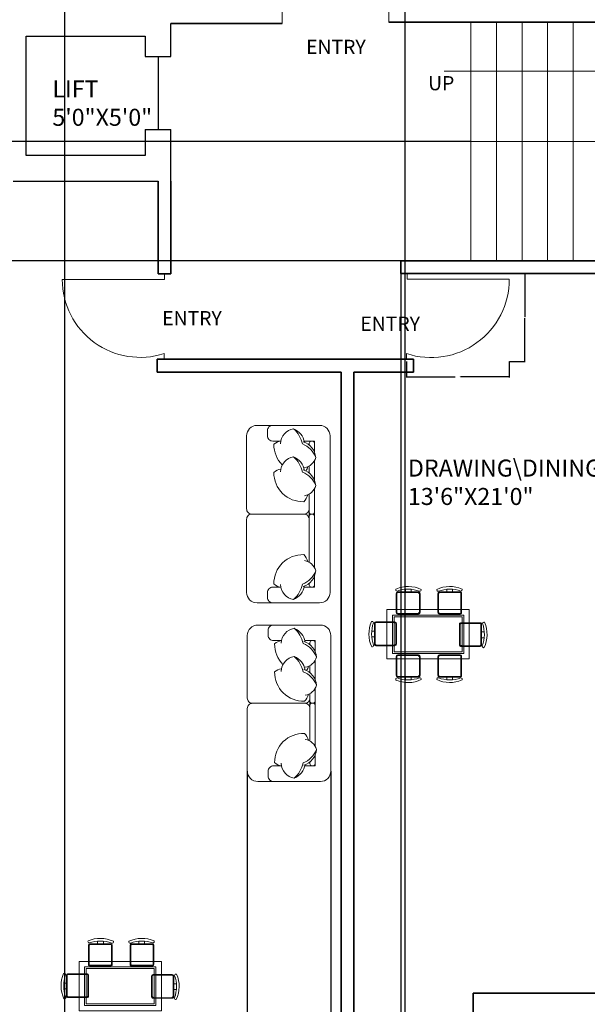
# Model space of a CAD drawing. Units: inches. Extents: x 1088 to 1703, y 668 to 1875.
# Tile 3 of 45: x 1302 to 1502, y 1069 to 1416. Entities that reach past the tile are written whole.
import ezdxf

# ---------------------------------------------------------------- set-up
doc = ezdxf.new("R2010")
doc.units = ezdxf.units.IN
for name, color, linetype, lineweight in [('A-ANNO-DIMS', 2, 'Continuous', 18), ('A-ANNO-SYMB', 7, 'Continuous', 18), ('A-ANNO-TEXT', 7, 'Continuous', 18), ('A-AREA-IDEN', 7, 'Continuous', 18), ('A-DOOR', 4, 'Continuous', 18), ('A-FLOR-EVTR', 5, 'Continuous', 25), ('A-FLOR-STRS', 7, 'Continuous', 18), ('A-FURN', 8, 'Continuous', 13), ('A-WALL', 7, 'Continuous', 35)]:
    doc.layers.add(name, color=color, linetype=linetype, lineweight=lineweight)
doc.styles.get("Standard").update_dxf_attribs({"font": 'arial.ttf'})
doc.dimstyles.get("Standard").update_dxf_attribs({"dimtxt": 0.18, "dimasz": 0.18, "dimexe": 0.18, "dimexo": 0.0625, "dimgap": 0.09, "dimtad": 0, "dimtih": 1, "dimtoh": 1, "dimdec": 4, "dimzin": 0, "dimdsep": 46, "dimtxsty": 'Standard', "dimcen": 0.09, "dimadec": 0, "dimazin": 0, "dimtfac": 1, "dimtdec": 4, "dimtofl": 0, "dimtmove": 0, "dimatfit": 3, "dimfxl": 1, "dimtolj": 1, "dimtzin": 0, "dimarcsym": 0})

# ---------------------------------------------------------------- blocks, each defined once
blk = doc.blocks.new('TABLE-DINING-RECT')
for points in [[(0, 17.41), (29.01, 17.41), (29.01, 0), (0, 0)], [(1.93, 15.47), (27.08, 15.47), (27.08, 1.93), (1.93, 1.93)], [(2.51, 14.89), (26.5, 14.89), (26.5, 2.51), (2.51, 2.51)]]:
    blk.add_lwpolyline(points, close=True)
blk = doc.blocks.new('CHAIR-DINING')
for points in [[(7.77, 8.29, 0.414214), (7.26, 8.81), (0.51, 8.81, 0.414214), (0, 8.29), (0, 0.96, 0.414214), (0.51, 0.44), (7.26, 0.44, 0.414214), (7.77, 0.96), (7.77, 8.29)], [(8.09, 8.52, -0.175809), (8.03, 0.62, 0.578392), (8.69, 0.02, 0.214524), (8.81, 8.94, 0.552014), (8.09, 8.52, -0.065079)], [(7.77, 3.53), (8.7, 3.53, -0.064759)]]:
    blk.add_lwpolyline(points, format="xyb")
blk.add_lwpolyline([(7.54, 8.29), (7.54, 1.19, -0.414214), (7.03, 0.68), (0.74, 0.68, -0.414214), (0.23, 1.19), (0.23, 8.29, -0.512069), (0.74, 8.58), (7.03, 8.58, -0.512069)], format="xyb", close=True)
blk.add_lwpolyline([(8.72, 5.59), (7.77, 5.59)])
blk = doc.blocks.new('DOOR-SWING-36')
for p, q in [((36.2, 30.23), (36.2, 28.23)), ((36, 2), (0, 2)), ((36, 0), (36, 2))]:
    blk.add_line(p, q)
blk.add_arc((27.61, 2), 27.61, 71.8583, 180)
blk = doc.blocks.new('*D26')
at = {"layer": 'A-ANNO-DIMS', "color": 0, "lineweight": -2, "transparency": 16777216}
for p, q in [((1437.89, 1295.51), (1437.89, 1289.96)), ((1474.09, 1295.51), (1474.09, 1289.96)), ((1438.07, 1290.14), (1455.06, 1290.14)), ((1473.91, 1290.14), (1456.93, 1290.14))]:
    blk.add_line(p, q, dxfattribs=at)
at = {"layer": 'A-ANNO-DIMS', "color": 0, "transparency": 16777216}
for points in [[(1438.07, 1290.17), (1438.07, 1290.11), (1437.89, 1290.14)], [(1473.91, 1290.17), (1473.91, 1290.11), (1474.09, 1290.14)]]:
    blk.add_solid(points, dxfattribs=at)
at = {"layer": 'Defpoints', "color": 0, "transparency": 16777216}
for p in [(1437.89, 1295.57), (1474.09, 1295.57), (1437.89, 1290.14)]:
    blk.add_point(p, dxfattribs=at)
at = {"layer": 'A-ANNO-DIMS', "color": 0, "transparency": 16777216, "insert": (1455.99, 1290.14), "char_height": 0.18, "attachment_point": 5}
blk.add_mtext('\\A1;DOOR 36 TYP.', dxfattribs=at)
blk = doc.blocks.new('*D27')
at = {"layer": 'A-ANNO-DIMS', "color": 0, "lineweight": -2, "transparency": 16777216}
for p, q in [((1474.16, 1326.56), (1479.71, 1326.56)), ((1479.53, 1326.38), (1479.53, 1311.25)), ((1479.53, 1295.75), (1479.53, 1310.88)), ((1474.16, 1295.57), (1479.71, 1295.57))]:
    blk.add_line(p, q, dxfattribs=at)
at = {"layer": 'A-ANNO-DIMS', "color": 0, "transparency": 16777216}
for points in [[(1479.5, 1326.38), (1479.56, 1326.38), (1479.53, 1326.56)], [(1479.5, 1295.75), (1479.56, 1295.75), (1479.53, 1295.57)]]:
    blk.add_solid(points, dxfattribs=at)
at = {"layer": 'Defpoints', "color": 0, "transparency": 16777216}
for p in [(1474.1, 1326.56), (1474.09, 1295.57), (1479.53, 1295.57)]:
    blk.add_point(p, dxfattribs=at)
at = {"layer": 'A-ANNO-DIMS', "color": 0, "transparency": 16777216, "insert": (1479.53, 1311.06), "char_height": 0.18, "attachment_point": 5}
blk.add_mtext('\\A1;31 TYP.', dxfattribs=at)
blk = doc.blocks.new('*D31')
at = {"layer": 'A-ANNO-DIMS', "color": 0, "lineweight": -2, "transparency": 16777216}
for p, q in [((1435.84, 1326.5), (1435.84, 725.55)), ((1585.84, 1326.5), (1585.84, 725.55)), ((1436.02, 725.73), (1510.56, 725.73)), ((1585.66, 725.73), (1511.12, 725.73))]:
    blk.add_line(p, q, dxfattribs=at)
at = {"layer": 'A-ANNO-DIMS', "color": 0, "transparency": 16777216}
for points in [[(1436.02, 725.76), (1436.02, 725.7), (1435.84, 725.73)], [(1585.66, 725.76), (1585.66, 725.7), (1585.84, 725.73)]]:
    blk.add_solid(points, dxfattribs=at)
at = {"layer": 'Defpoints', "color": 0, "transparency": 16777216}
for p in [(1435.84, 1326.56), (1585.84, 1326.56), (1585.84, 725.73)]:
    blk.add_point(p, dxfattribs=at)
at = {"layer": 'A-ANNO-DIMS', "color": 0, "transparency": 16777216, "insert": (1510.84, 725.73), "char_height": 0.18, "attachment_point": 5}
blk.add_mtext('\\A1;150', dxfattribs=at)
blk = doc.blocks.new('*D34')
at = {"layer": 'A-ANNO-DIMS', "color": 0, "lineweight": -2, "transparency": 16777216}
for p, q in [((1460.53, 1373.06), (1116.11, 1373.06)), ((1116.29, 1372.88), (1116.29, 1352.24)), ((1116.29, 1331.24), (1116.29, 1351.88)), ((1460.53, 1331.06), (1116.11, 1331.06))]:
    blk.add_line(p, q, dxfattribs=at)
at = {"layer": 'A-ANNO-DIMS', "color": 0, "transparency": 16777216}
for points in [[(1116.26, 1372.88), (1116.32, 1372.88), (1116.29, 1373.06)], [(1116.26, 1331.24), (1116.32, 1331.24), (1116.29, 1331.06)]]:
    blk.add_solid(points, dxfattribs=at)
at = {"layer": 'Defpoints', "color": 0, "transparency": 16777216}
for p in [(1116.29, 1373.06), (1460.59, 1373.06), (1460.59, 1331.06)]:
    blk.add_point(p, dxfattribs=at)
at = {"layer": 'A-ANNO-DIMS', "color": 0, "transparency": 16777216, "insert": (1116.29, 1352.06), "char_height": 0.18, "attachment_point": 5}
blk.add_mtext('\\A1;42', dxfattribs=at)
blk = doc.blocks.new('*D37')
at = {"layer": 'A-ANNO-DIMS', "color": 0, "lineweight": -2, "transparency": 16777216}
for p, q in [((1381.79, 1151.2), (1381.79, 725.55)), ((1411.2, 1151.2), (1411.2, 725.55)), ((1381.97, 725.73), (1396.11, 725.73)), ((1411.02, 725.73), (1396.87, 725.73))]:
    blk.add_line(p, q, dxfattribs=at)
at = {"layer": 'A-ANNO-DIMS', "color": 0, "transparency": 16777216}
for points in [[(1381.97, 725.76), (1381.97, 725.7), (1381.79, 725.73)], [(1411.02, 725.76), (1411.02, 725.7), (1411.2, 725.73)]]:
    blk.add_solid(points, dxfattribs=at)
at = {"layer": 'Defpoints', "color": 0, "transparency": 16777216}
for p in [(1381.79, 1151.26), (1411.2, 1151.26), (1411.2, 725.73)]:
    blk.add_point(p, dxfattribs=at)
at = {"layer": 'A-ANNO-DIMS', "color": 0, "transparency": 16777216, "insert": (1396.49, 725.73), "char_height": 0.18, "attachment_point": 5}
blk.add_mtext('\\A1;29.41', dxfattribs=at)
blk = doc.blocks.new('*D38')
at = {"layer": 'A-ANNO-DIMS', "color": 0, "lineweight": -2, "transparency": 16777216}
for p, q in [((1317.34, 1736.94), (1317.34, 725.55)), ((1437.34, 1736.94), (1437.34, 725.55)), ((1317.52, 725.73), (1377.06, 725.73)), ((1437.16, 725.73), (1377.62, 725.73))]:
    blk.add_line(p, q, dxfattribs=at)
at = {"layer": 'A-ANNO-DIMS', "color": 0, "transparency": 16777216}
for points in [[(1317.52, 725.76), (1317.52, 725.7), (1317.34, 725.73)], [(1437.16, 725.76), (1437.16, 725.7), (1437.34, 725.73)]]:
    blk.add_solid(points, dxfattribs=at)
at = {"layer": 'Defpoints', "color": 0, "transparency": 16777216}
for p in [(1317.34, 1737.01), (1437.34, 1737.01), (1437.34, 725.73)]:
    blk.add_point(p, dxfattribs=at)
at = {"layer": 'A-ANNO-DIMS', "color": 0, "transparency": 16777216, "insert": (1377.34, 725.73), "char_height": 0.18, "attachment_point": 5}
blk.add_mtext('\\A1;120', dxfattribs=at)

msp = doc.modelspace()

# ---------------------------------------------------------------- linework, layer by layer
at = {"layer": 'A-ANNO-SYMB'}
msp.add_line((1451.148, 1397.817), (1569.925, 1397.817), dxfattribs=at)
at = {"layer": 'A-DOOR'}
for p, q in [((1394.044, 1419.144), (1394.044, 1414.644)), ((1431.608, 1415.058), (1431.608, 1419.558)), ((1352.595, 1326.469), (1352.595, 1324.469)), ((1352.595, 1324.469), (1316.595, 1324.469)), ((1352.476, 1296.327), (1352.476, 1298.327))]:
    msp.add_line(p, q, dxfattribs=at)
msp.add_arc((1344.058, 1324.469), 27.463, 180, 287.84855, dxfattribs=at)
at = {"layer": 'A-FLOR-EVTR'}
for p, q in [((1354.845, 1403.022), (1354.845, 1414.644)), ((1303.845, 1410.144), (1345.845, 1410.144)), ((1303.845, 1368.144), (1303.845, 1410.144)), ((1345.845, 1410.144), (1345.845, 1403.022)), ((1345.845, 1403.022), (1354.845, 1403.022)), ((1350.345, 1403.022), (1350.345, 1377.328)), ((1345.845, 1377.328), (1354.845, 1377.328)), ((1345.845, 1377.328), (1345.845, 1368.144)), ((1354.845, 1359.144), (1354.845, 1377.328)), ((1345.845, 1368.144), (1303.845, 1368.144)), ((1299.345, 1359.144), (1350.345, 1359.144))]:
    msp.add_line(p, q, dxfattribs=at)
at = {"layer": 'A-FLOR-STRS'}
for p, q in [((1460.595, 1415.058), (1460.595, 1331.058)), ((1469.595, 1415.058), (1469.595, 1331.058)), ((1478.595, 1415.058), (1478.595, 1331.058)), ((1487.595, 1415.058), (1487.595, 1331.058)), ((1496.595, 1415.058), (1496.595, 1331.058)), ((1460.595, 1331.058), (1460.595, 1373.058)), ((1460.595, 1373.058), (1550.595, 1373.058))]:
    msp.add_line(p, q, dxfattribs=at)
at = {"layer": 'A-FURN', "ltscale": 0.03}
for points in [[(1381.539, 1239.954, -0.4142136), (1383.378, 1241.792, -0.4142136), (1381.539, 1243.63), (1381.539, 1269.365, -0.4142136), (1385.216, 1273.041), (1407.274, 1273.041, -0.4142136), (1410.951, 1269.365), (1410.951, 1214.219, -0.4142136), (1407.274, 1210.542), (1385.216, 1210.542, -0.4142136), (1381.539, 1214.219), (1381.539, 1239.954, -0.4142136), (1383.378, 1241.792, -0.4142136), (1381.539, 1243.63)], [(1381.786, 1173.318, -0.4142136), (1383.625, 1175.156, -0.4142136), (1381.786, 1176.994), (1381.786, 1199.053, -0.4142136), (1385.463, 1202.729), (1407.521, 1202.729, -0.4142136), (1411.198, 1199.053), (1411.198, 1151.259, -0.4142136), (1407.521, 1147.583), (1385.463, 1147.583, -0.4142136), (1381.786, 1151.259), (1381.786, 1173.318, -0.4142136), (1383.625, 1175.156, -0.4142136), (1381.786, 1176.994)]]:
    msp.add_lwpolyline(points, format="xyb", dxfattribs=at)
at = {"layer": 'A-FURN'}
for points in [[(1393.579, 1267.527), (1390.73, 1267.527, -0.4142136), (1388.892, 1269.365), (1388.892, 1271.203, -0.4142136), (1390.73, 1273.041)], [(1393.467, 1266.604, -0.3567724), (1398.101, 1271.872, -0.2495421), (1401.919, 1267.099, 9.6168803)], [(1398.101, 1271.872, -0.1477299), (1401.26, 1266.499, -0.2133428), (1405.893, 1261.758, -0.1786618)], [(1393.579, 1267.531, 0.1655406), (1391.151, 1266.394, 0.2002311), (1394.109, 1259.097, 0.1215233)], [(1401.512, 1267.241, -0.3066635), (1405.893, 1261.758, -0.30633), (1401.892, 1258.177, 0.8728472)], [(1405.436, 1263.66), (1405.436, 1267.527), (1401.824, 1267.527, -0.4142136)], [(1403.598, 1266.124), (1403.598, 1266.792, -0.4142136), (1404.333, 1267.527), (1404.701, 1267.527, -0.4142136), (1405.436, 1266.792)], [(1405.436, 1266.792), (1405.436, 1263.66, -0.4142136)], [(1393.467, 1256.702, -0.3567724), (1398.101, 1261.969, -0.2495421), (1401.919, 1257.197, 9.6168803)], [(1398.101, 1261.969, -0.1477299), (1401.26, 1256.597, -0.2133428), (1405.893, 1251.856, -0.1786618)], [(1405.436, 1260.602), (1405.436, 1253.757, -0.4142136)], [(1393.579, 1257.628, 0.1655406), (1391.151, 1256.491, 0.4259892), (1401.681, 1246.168, 0.1215233), (1403.133, 1248.618, -7.1154643)], [(1401.512, 1257.339, -0.3066635), (1405.893, 1251.856, -0.30633), (1401.892, 1248.274, 0.8728472)], [(1402.414, 1256.979, 0.0718654), (1403.133, 1258.521, -7.1154643)], [(1403.598, 1256.222), (1403.598, 1258.751, -0.4142136)], [(1405.436, 1250.699), (1405.436, 1242.527, -0.4142136), (1404.701, 1241.792), (1404.333, 1241.792, -0.4142136), (1403.598, 1242.527), (1403.598, 1248.848, -0.4142136)], [(1403.598, 1243.63, -0.4142136), (1401.76, 1241.792), (1383.378, 1241.792, -0.4142136)], [(1403.598, 1243.63, -0.4142136), (1401.76, 1241.792)], [(1403.598, 1239.954, 0.4142136), (1401.76, 1241.792), (1383.378, 1241.792, 0.4142136)], [(1403.598, 1239.954, 0.4142136), (1401.76, 1241.792)], [(1405.436, 1222.982), (1405.436, 1241.057, 0.4142136), (1404.701, 1241.792), (1404.333, 1241.792, 0.4142136), (1403.598, 1241.057), (1403.598, 1224.833, 0.4142136)], [(1393.579, 1216.053, -0.1655406), (1391.151, 1217.19, -0.4259892), (1401.681, 1227.514, -0.1215233), (1403.133, 1225.063, 7.1154643)], [(1401.512, 1216.343, 0.3066635), (1405.893, 1221.825, 0.30633), (1401.892, 1225.407, -0.8728472)], [(1398.101, 1211.712, 0.1477299), (1401.26, 1217.085, 0.2133428), (1405.893, 1221.825, 0.1786618)], [(1405.436, 1216.792), (1405.436, 1219.924, 0.4142136)], [(1390.73, 1210.542, -0.4142136), (1388.892, 1212.381), (1388.892, 1214.219, -0.4142136), (1390.73, 1216.057), (1393.579, 1216.057)], [(1393.467, 1216.979, 0.3567724), (1398.101, 1211.712, 0.2495421), (1401.919, 1216.485, -9.6168803)], [(1403.598, 1217.46), (1403.598, 1216.792, 0.4142136), (1404.333, 1216.057), (1404.701, 1216.057, 0.4142136), (1405.436, 1216.792)], [(1434.566, 1214.69, -0.1758092), (1442.468, 1214.63, 0.5783921), (1443.067, 1215.288, 0.2145244), (1434.147, 1215.408, 0.552014), (1434.566, 1214.69, -0.065079)], [(1442.133, 1214.373), (1434.797, 1214.373, 0.4142136), (1434.284, 1213.86), (1434.284, 1207.115, 0.4142136), (1434.797, 1206.601), (1442.133, 1206.601, 0.4142136), (1442.646, 1207.115), (1442.646, 1213.86, 0.4142136), (1442.133, 1214.373)], [(1439.556, 1214.373), (1439.556, 1215.301, -0.0647586)], [(1449.12, 1214.63, -0.5783921), (1448.522, 1215.288, -0.2145244), (1457.441, 1215.408, -0.552014), (1457.022, 1214.69, 0.1758092), (1449.12, 1214.63)], [(1456.791, 1214.373, -0.4142136), (1457.304, 1213.86), (1457.304, 1207.115, -0.4142136), (1456.791, 1206.601), (1449.456, 1206.601, -0.4142136), (1448.942, 1207.115), (1448.942, 1213.86, -0.4142136), (1449.456, 1214.373), (1456.791, 1214.373)], [(1452.032, 1214.373), (1452.032, 1215.301, 0.0647586)], [(1426.3, 1195.609, -0.5783921), (1425.641, 1195.01, -0.2145244), (1425.522, 1203.929, -0.552014), (1426.24, 1203.51, 0.1758094), (1426.3, 1195.609)], [(1426.557, 1203.28, -0.4142136), (1427.07, 1203.793), (1433.815, 1203.793, -0.4142136), (1434.328, 1203.28), (1434.328, 1195.944, -0.4142136), (1433.815, 1195.431), (1427.07, 1195.431, -0.4142136), (1426.557, 1195.944), (1426.557, 1203.28)], [(1393.825, 1197.214), (1390.977, 1197.214, -0.4142136), (1389.139, 1199.053), (1389.139, 1200.891, -0.4142136), (1390.977, 1202.729)], [(1393.714, 1196.292, -0.3567724), (1398.348, 1201.559, -0.2495421), (1402.166, 1196.787, 9.6168803)], [(1398.348, 1201.559, -0.1477299), (1401.507, 1196.187, -0.2133428), (1406.14, 1191.446, -0.1786618)], [(1393.826, 1197.218, 0.1655406), (1391.398, 1196.081, 0.2002311), (1394.356, 1188.784, 0.1215233)], [(1401.759, 1196.929, -0.3066635), (1406.14, 1191.446, -0.30633), (1402.139, 1187.864, 0.8728472)], [(1405.683, 1193.347), (1405.683, 1197.214), (1402.071, 1197.214, -0.4142136)], [(1403.845, 1195.812), (1403.845, 1196.479, -0.4142136), (1404.58, 1197.214), (1404.948, 1197.214, -0.4142136), (1405.683, 1196.479)], [(1426.557, 1198.521), (1425.629, 1198.521, 0.0647586)], [(1405.683, 1196.479), (1405.683, 1193.347, -0.4142136)], [(1393.714, 1186.39, -0.3567724), (1398.348, 1191.657, -0.2495421), (1402.166, 1186.884, 9.6168803)], [(1398.348, 1191.657, -0.1477299), (1401.507, 1186.284, -0.2133428), (1406.14, 1181.544, -0.1786618)], [(1405.683, 1190.289), (1405.683, 1183.445, -0.4142136)], [(1456.791, 1184.39, 0.4142136), (1457.304, 1184.903), (1457.304, 1191.648, 0.4142136), (1456.791, 1192.161), (1449.456, 1192.161, 0.4142136), (1448.942, 1191.648), (1448.942, 1184.903, 0.4142136), (1449.456, 1184.39), (1456.791, 1184.39)], [(1393.826, 1187.316, 0.1655406), (1391.398, 1186.179, 0.4259892), (1401.928, 1175.855, 0.1215233), (1403.379, 1178.306, -7.1154643)], [(1401.759, 1187.026, -0.3066635), (1406.14, 1181.544, -0.30633), (1402.139, 1177.962, 0.8728472)], [(1402.661, 1186.667, 0.0718654), (1403.379, 1188.208, -7.1154643)], [(1403.845, 1185.909), (1403.845, 1188.438, -0.4142136)], [(1457.022, 1184.073, -0.1758093), (1449.12, 1184.132, 0.5783921), (1448.522, 1183.474, 0.2145244), (1457.441, 1183.354, 0.552014), (1457.022, 1184.073, -0.065079)], [(1452.032, 1184.39), (1452.032, 1183.462, -0.0647586)], [(1405.683, 1180.387), (1405.683, 1175.891, -0.4142136), (1404.948, 1175.156), (1404.58, 1175.156, -0.4142136), (1403.845, 1175.891), (1403.845, 1178.536, -0.4142136)], [(1403.845, 1176.994, -0.4142136), (1402.007, 1175.156), (1383.625, 1175.156, -0.4142136)], [(1403.845, 1176.994, -0.4142136), (1402.007, 1175.156)], [(1403.845, 1173.318, 0.4142136), (1402.007, 1175.156), (1383.625, 1175.156, 0.4142136)], [(1403.845, 1173.318, 0.4142136), (1402.007, 1175.156)], [(1405.683, 1160.023), (1405.683, 1174.421, 0.4142136), (1404.948, 1175.156), (1404.58, 1175.156, 0.4142136), (1403.845, 1174.421), (1403.845, 1161.874, 0.4142136)], [(1393.826, 1153.093, -0.1655406), (1391.398, 1154.231, -0.4259892), (1401.928, 1164.554, -0.1215233), (1403.379, 1162.104, 7.1154643)], [(1401.759, 1153.383, 0.3066635), (1406.14, 1158.866, 0.30633), (1402.139, 1162.447, -0.8728472)], [(1398.348, 1148.753, 0.1477299), (1401.507, 1154.125, 0.2133428), (1406.14, 1158.866, 0.1786618)], [(1405.683, 1153.833), (1405.683, 1156.964, 0.4142136)], [(1390.977, 1147.583, -0.4142136), (1389.139, 1149.421), (1389.139, 1151.259, -0.4142136), (1390.977, 1153.097), (1393.825, 1153.097)], [(1393.714, 1154.02, 0.3567724), (1398.348, 1148.753, 0.2495421), (1402.166, 1153.525, -9.6168803)], [(1403.845, 1154.5), (1403.845, 1153.833, 0.4142136), (1404.58, 1153.097), (1404.948, 1153.097, 0.4142136), (1405.683, 1153.833)], [(1326.098, 1090.719, -0.1758092), (1334, 1090.659, 0.5783921), (1334.598, 1091.317, 0.2145244), (1325.679, 1091.437, 0.552014), (1326.098, 1090.719, -0.065079)], [(1333.664, 1090.402), (1326.329, 1090.402, 0.4142136), (1325.816, 1089.889), (1325.816, 1083.144, 0.4142136), (1326.329, 1082.63), (1333.664, 1082.63, 0.4142136), (1334.178, 1083.144), (1334.178, 1089.889, 0.4142136), (1333.664, 1090.402)], [(1331.088, 1090.402), (1331.088, 1091.33, -0.0647586)], [(1340.652, 1090.659, -0.5783921), (1340.053, 1091.317, -0.2145244), (1348.973, 1091.437, -0.552014), (1348.554, 1090.719, 0.1758092), (1340.652, 1090.659)], [(1348.323, 1090.402, -0.4142136), (1348.836, 1089.889), (1348.836, 1083.144, -0.4142136), (1348.323, 1082.63), (1340.987, 1082.63, -0.4142136), (1340.474, 1083.144), (1340.474, 1089.889, -0.4142136), (1340.987, 1090.402), (1348.323, 1090.402)], [(1343.564, 1090.402), (1343.564, 1091.33, 0.0647586)], [(1317.831, 1071.638, -0.5783921), (1317.173, 1071.039, -0.2145244), (1317.053, 1079.958, -0.552014), (1317.771, 1079.539, 0.1758094), (1317.831, 1071.638)], [(1318.089, 1079.308, -0.4142136), (1318.602, 1079.822), (1325.347, 1079.822, -0.4142136), (1325.86, 1079.308), (1325.86, 1071.973, -0.4142136), (1325.347, 1071.46), (1318.602, 1071.46, -0.4142136), (1318.089, 1071.973), (1318.089, 1079.308)], [(1355.864, 1079.057, 0.4142136), (1355.351, 1079.57), (1348.606, 1079.57, 0.4142136), (1348.092, 1079.057), (1348.092, 1071.722, 0.4142136), (1348.606, 1071.208), (1355.351, 1071.208, 0.4142136), (1355.864, 1071.722), (1355.864, 1079.057)], [(1356.181, 1079.288, -0.1758092), (1356.121, 1071.386, 0.5783921), (1356.779, 1070.788, 0.2145244), (1356.899, 1079.707, 0.552014), (1356.181, 1079.288, -0.065079)], [(1318.089, 1074.549), (1317.161, 1074.549, 0.0647586)], [(1355.864, 1074.298), (1356.792, 1074.298, -0.0647586)]]:
    msp.add_lwpolyline(points, format="xyb", dxfattribs=at)
for points in [[(1405.436, 1253.757), (1405.436, 1260.602)], [(1405.436, 1222.982), (1405.436, 1250.699)], [(1401.824, 1216.057), (1405.436, 1216.057), (1405.436, 1219.924)], [(1437.503, 1215.317), (1437.503, 1214.373)], [(1454.086, 1215.317), (1454.086, 1214.373)], [(1425.612, 1200.574), (1426.557, 1200.574)], [(1405.683, 1183.445), (1405.683, 1190.289)], [(1454.086, 1183.445), (1454.086, 1184.39)], [(1405.683, 1160.023), (1405.683, 1180.387)], [(1402.071, 1153.097), (1405.683, 1153.097), (1405.683, 1156.964)], [(1329.034, 1091.346), (1329.034, 1090.402)], [(1345.617, 1091.346), (1345.617, 1090.402)], [(1317.144, 1076.603), (1318.089, 1076.603)], [(1356.808, 1076.352), (1355.864, 1076.352)]]:
    msp.add_lwpolyline(points, dxfattribs=at)
for points in [[(1405.436, 1241.057), (1405.436, 1242.527, -0.4142136), (1404.701, 1241.792), (1404.333, 1241.792, -0.4142136), (1403.598, 1242.527), (1403.598, 1241.057, -0.4142136), (1404.333, 1241.792), (1404.701, 1241.792, -0.4142136)], [(1434.8, 1214.142), (1441.902, 1214.142, -0.4142136), (1442.415, 1213.628), (1442.415, 1207.346, -0.4142136), (1441.902, 1206.833), (1434.8, 1206.833, -0.5120695), (1434.515, 1207.346), (1434.515, 1213.628, -0.5120695)], [(1456.788, 1214.142), (1449.687, 1214.142, 0.4142136), (1449.174, 1213.628), (1449.174, 1207.346, 0.4142136), (1449.687, 1206.833), (1456.788, 1206.833, 0.5120695), (1457.073, 1207.346), (1457.073, 1213.628, 0.5120695)], [(1426.788, 1203.276), (1426.788, 1196.175, 0.4142136), (1427.301, 1195.662), (1433.584, 1195.662, 0.4142136), (1434.097, 1196.175), (1434.097, 1203.276, 0.5120695), (1433.584, 1203.562), (1427.301, 1203.562, 0.5120695)], [(1456.788, 1184.621), (1449.687, 1184.621, -0.4142136), (1449.174, 1185.134), (1449.174, 1191.417, -0.4142136), (1449.687, 1191.93), (1456.788, 1191.93, -0.5120695), (1457.073, 1191.417), (1457.073, 1185.134, -0.5120695)], [(1405.683, 1174.421), (1405.683, 1175.891, -0.4142136), (1404.948, 1175.156), (1404.58, 1175.156, -0.4142136), (1403.845, 1175.891), (1403.845, 1174.421, -0.4142136), (1404.58, 1175.156), (1404.948, 1175.156, -0.4142136)], [(1326.332, 1090.171), (1333.433, 1090.171, -0.4142136), (1333.946, 1089.657), (1333.946, 1083.375, -0.4142136), (1333.433, 1082.862), (1326.332, 1082.862, -0.5120695), (1326.047, 1083.375), (1326.047, 1089.657, -0.5120695)], [(1348.32, 1090.171), (1341.218, 1090.171, 0.4142136), (1340.705, 1089.657), (1340.705, 1083.375, 0.4142136), (1341.218, 1082.862), (1348.32, 1082.862, 0.5120695), (1348.605, 1083.375), (1348.605, 1089.657, 0.5120695)], [(1318.32, 1079.305), (1318.32, 1072.204, 0.4142136), (1318.833, 1071.691), (1325.116, 1071.691, 0.4142136), (1325.629, 1072.204), (1325.629, 1079.305, 0.5120695), (1325.116, 1079.59), (1318.833, 1079.59, 0.5120695)], [(1355.633, 1079.054), (1355.633, 1071.953, -0.4142136), (1355.119, 1071.44), (1348.837, 1071.44, -0.4142136), (1348.324, 1071.953), (1348.324, 1079.054, -0.5120695), (1348.837, 1079.339), (1355.119, 1079.339, -0.5120695)]]:
    msp.add_lwpolyline(points, format="xyb", close=True, dxfattribs=at)
at = {"layer": 'A-WALL'}
for p, q in [((1394.044, 1414.644), (1354.845, 1414.644)), ((1431.608, 1415.058), (1435.845, 1415.058)), ((1435.845, 1415.058), (1431.608, 1415.058)), ((1485.345, 1415.058), (1435.845, 1415.058)), ((1435.845, 1415.058), (1440.345, 1415.058)), ((1485.345, 1415.058), (1590.345, 1415.058)), ((1350.345, 1342.503), (1350.345, 1359.144)), ((1354.845, 1359.144), (1354.845, 1342.503)), ((1350.345, 1342.503), (1350.345, 1326.469)), ((1354.845, 1326.469), (1354.845, 1345.129)), ((1435.845, 1331.058), (1585.845, 1331.058)), ((1435.845, 1331.058), (1435.845, 1326.558)), ((1350.345, 1326.469), (1354.845, 1326.469)), ((1435.845, 1326.558), (1585.845, 1326.558)), ((1435.845, 1326.558), (1440.345, 1326.558)), ((1419.345, 1296.327), (1350.029, 1296.327)), ((1350.029, 1296.327), (1350.029, 1291.827)), ((1419.345, 1296.327), (1414.845, 1296.327)), ((1440.345, 1296.327), (1419.345, 1296.327)), ((1440.345, 1291.827), (1440.345, 1296.327)), ((1350.029, 1291.827), (1414.845, 1291.827)), ((1414.845, 1291.827), (1414.845, 1027.308)), ((1419.345, 965.058), (1419.345, 1291.827)), ((1419.345, 1291.827), (1440.345, 1291.827)), ((1414.845, 1154.058), (1414.845, 969.558)), ((1419.345, 965.058), (1419.345, 1154.058)), ((1461.345, 1073.058), (1585.845, 1073.058)), ((1465.845, 1073.058), (1461.345, 1073.058)), ((1461.345, 1073.058), (1461.345, 1040.808))]:
    msp.add_line(p, q, dxfattribs=at)

# ---------------------------------------------------------------- block references
at = {"layer": 'A-DOOR', "rotation": 179.9986759845218}
msp.add_blockref('DOOR-SWING-36', (1474.096, 1326.559), dxfattribs=at)
at = {"layer": 'A-FURN'}
for name, p in [('TABLE-DINING-RECT', (1430.978, 1190.771)), ('CHAIR-DINING', (1456.561, 1194.735)), ('TABLE-DINING-RECT', (1322.51, 1066.8))]:
    msp.add_blockref(name, p, dxfattribs=at)
at = {"layer": 'A-FURN', "extrusion": (0, 0, -1), "zscale": -1, "rotation": 270.0000017090653}
msp.add_blockref('CHAIR-DINING', (-1443.09, 1192.161), dxfattribs=at)

# ---------------------------------------------------------------- texts
at = {"layer": 'A-ANNO-TEXT', "char_height": 5, "attachment_point": 1}
for s, width, insert in [('ENTRY', 23.80078, (1402.508, 1408.901)), ('UP', 12.41346, (1445.493, 1396.116)), ('ENTRY', 29.20961, (1351.802, 1313.326)), ('ENTRY', 20.23245, (1421.625, 1311.362))]:
    msp.add_mtext_dynamic_manual_height_columns(s, width=width, gutter_width=12.5, heights=[0], dxfattribs=dict(at, insert=insert))
at = {"layer": 'A-AREA-IDEN', "char_height": 6, "attachment_point": 1}
for s, width, insert in [('LIFT\\P5\'0"X5\'0"', 86.93639, (1313.103, 1394.599)), ('DRAWING\\\\DINING HALL\\P13\'6"X21\'0"', 91.5795, (1438.37, 1261.013))]:
    msp.add_mtext_dynamic_manual_height_columns(s, width=width, gutter_width=12.5, heights=[0], dxfattribs=dict(at, insert=insert))

# ---------------------------------------------------------------- dimensions: what is measured, and where the dimension line sits
at = {"layer": 'A-ANNO-DIMS'}
for base, p1, p2, override, picture, middle in [((1437.345, 725.729), (1317.345, 1737.007), (1437.345, 1737.007), {"dimdec": 0, "dimlfac": 1, "dimrnd": 0, "dimzin": 0, "dimdsep": 46, "dimlunit": 2}, '*D38', (1377.345, 725.729)), ((1585.845, 725.729), (1435.845, 1326.558), (1585.845, 1326.558), {"dimdec": 0, "dimlfac": 1, "dimrnd": 0, "dimzin": 0, "dimdsep": 46, "dimlunit": 2}, '*D31', (1510.845, 725.729)), ((1411.198, 725.729), (1381.786, 1151.259), (1411.198, 1151.259), {"dimdec": 2, "dimlfac": 1, "dimrnd": 0, "dimzin": 0, "dimdsep": 46, "dimlunit": 2}, '*D37', (1396.492, 725.729))]:
    dim = msp.add_linear_dim(base=base, p1=p1, p2=p2, dimstyle='Standard', override=override, dxfattribs=at)
    dim.commit()
    dim.dimension.update_dxf_attribs({"geometry": picture, "text_midpoint": middle})
dim = msp.add_linear_dim(base=(1116.295, 1373.058), p1=(1460.595, 1331.058), p2=(1460.595, 1373.058), angle=90, dimstyle='Standard', override={"dimdec": 0, "dimlfac": 1, "dimrnd": 0, "dimzin": 0, "dimdsep": 46, "dimlunit": 2}, dxfattribs=at)
dim.commit()
dim.dimension.update_dxf_attribs({"geometry": '*D34', "text_midpoint": (1116.295, 1352.058)})
for base, p1, p2, angle, text, picture, middle in [((1479.525, 1295.569), (1474.096, 1326.559), (1474.095, 1295.569), 269.99868, '<> TYP.', '*D27', (1479.526, 1311.064)), ((1437.893, 1290.14), (1474.095, 1295.569), (1437.893, 1295.57), 179.99868, 'DOOR <> TYP.', '*D26', (1455.994, 1290.14))]:
    dim = msp.add_linear_dim(base=base, p1=p1, p2=p2, angle=angle, text=text, dimstyle='Standard', override={"dimdec": 0, "dimlfac": 1, "dimrnd": 0, "dimzin": 0, "dimdsep": 46, "dimlunit": 2}, dxfattribs=at)
    dim.commit()
    dim.dimension.update_dxf_attribs({"geometry": picture, "text_midpoint": middle})

doc.saveas('drawing.dxf')
